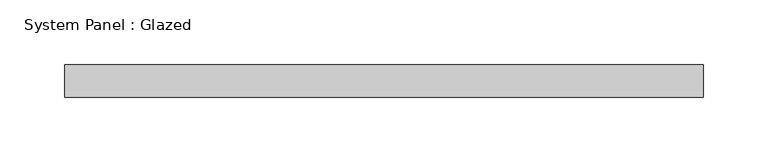
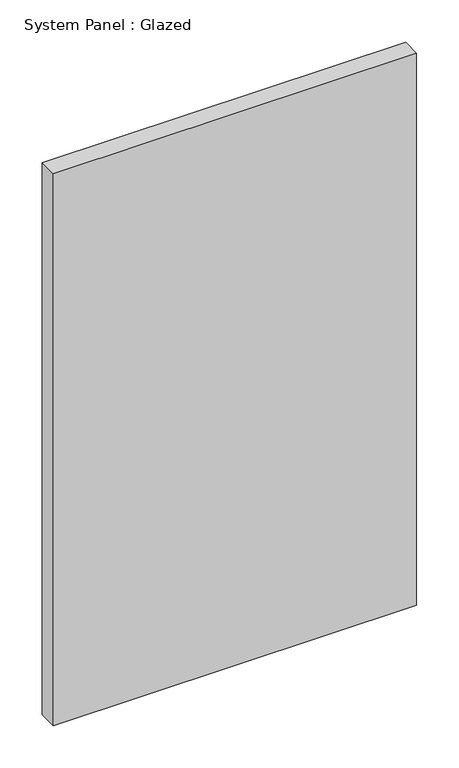
"""IFC4 building model written with IfcOpenShell, lengths in millimetres: plate geometry, System Panel : Glazed."""

from ifc_helpers import new_model, si_unit, origin, origin_with_axes, place, context, project, spatial, polyline, outline, extrude, source, transform, mapped, element, save


def system_panel_glazed_3330f8c4(model_context):
    return source(origin(), model_context, "Body", "SweptSolid", [
        extrude(outline(polyline([(247.65, 19.05), (-247.65, 19.05), (-247.65, 44.45), (247.65, 44.45), (247.65, 19.05)])), origin_with_axes(), (0.0, 0.0, 1.0), 794.5627727),
    ])


if __name__ == "__main__":
    model = new_model("IFC4")
    model_context = context("Model", 3, world=origin())
    ifc_project = project(units=[si_unit("LENGTHUNIT", "METRE", prefix="MILLI")], contexts=[model_context])
    site = spatial("IfcSite", under=ifc_project)
    building = spatial("IfcBuilding", under=site)
    placement = place(None, origin())
    system_panel_glazed_shape = system_panel_glazed_3330f8c4(model_context)
    element("IfcPlate", 1, ObjectType="System Panel : Glazed", at=placement, inside=building, context=model_context, shape_type="MappedRepresentation", body=[
        mapped(system_panel_glazed_shape, transform((0.0, 0.0, 0.0), x_axis=(1.0, 0.0, 0.0), y_axis=(0.0, 1.0, 0.0), z_axis=(0.0, 0.0, 1.0))),
    ])
    save(model, "model.ifc")

# Revit data of these elements
# Type "System Panel : Glazed"
#   Construction Type Id = "GSP4R"
#   Analytic Construction = "1/8 in Pilkington single glazing"
#   Visual Light Transmittance = 0.9
#   Solar Heat Gain Coefficient = 0.86
#   Heat Transfer Coefficient (U) = 1.18115 BTU/(h·ft²·°F)
#   Define Thermal Properties by = 1
# Element 1 (IfcPlate, "System Panel : Glazed")
#   Materials on its faces: "Glass"
# Materials
#   "Glass": class "Glass", colour RGB 0 128 192, transparency 0.75, Description = "Soda Lime Glass", Cost = 0
